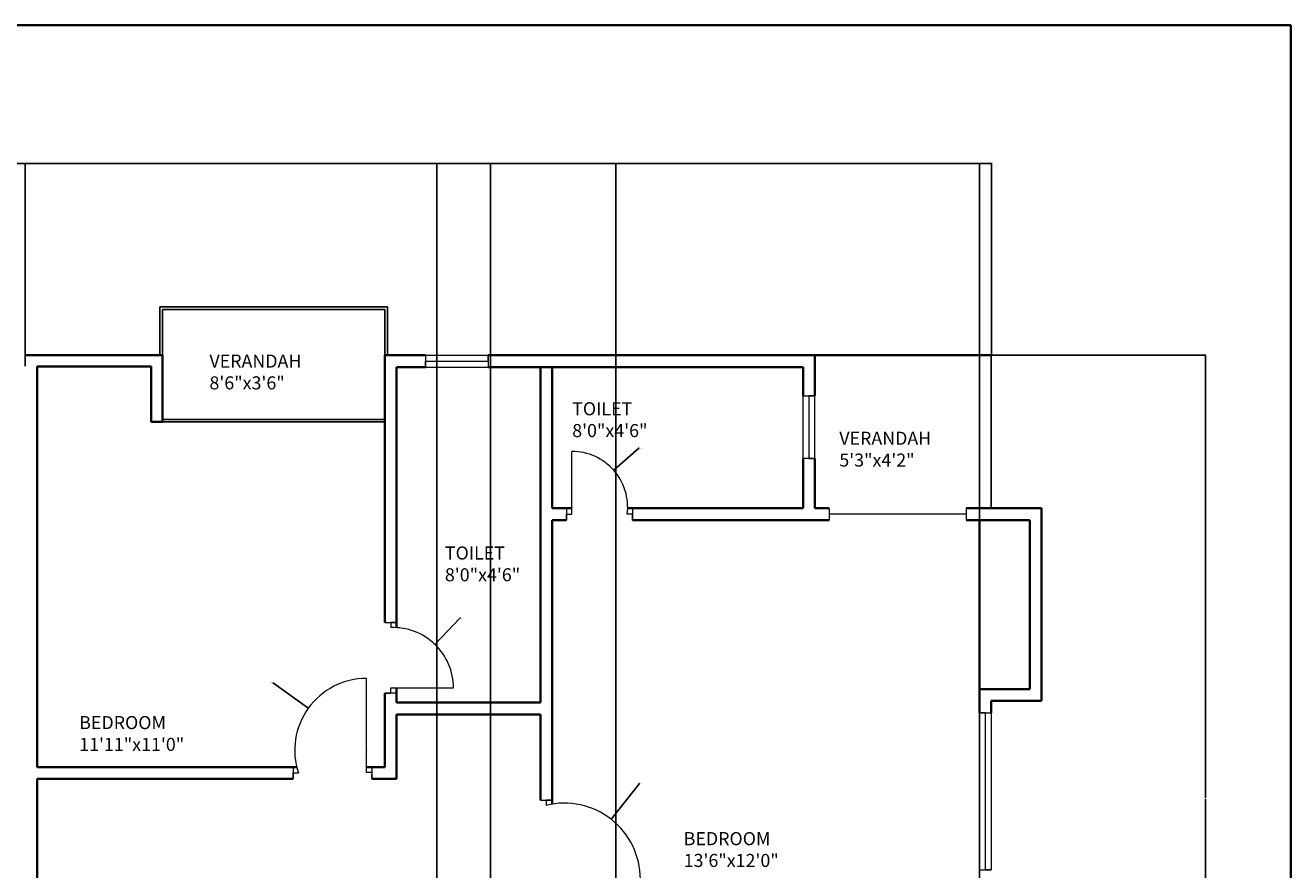
# Model space of a CAD drawing. Units: inches. Extents: x 2154 to 3131, y 1384 to 2688.
# Tile 5 of 5: x 2647 to 3131, y 2365 to 2688. Entities that reach past the tile are written whole.
import ezdxf

# ---------------------------------------------------------------- set-up
doc = ezdxf.new("R2010")
doc.units = ezdxf.units.IN
for name, color, linetype, lineweight in [('A-ANNO-DIMS', 2, 'Continuous', 18), ('A-ANNO-TTLB', 7, 'Continuous', 35), ('A-AREA-IDEN', 7, 'Continuous', 18), ('A-DOOR', 31, 'Continuous', 18), ('A-FLOR-BALC', 130, 'Continuous', 25), ('A-GLAZ', 130, 'Continuous', 18), ('A-WALL', 7, 'Continuous', 35)]:
    doc.layers.add(name, color=color, linetype=linetype, lineweight=lineweight)
doc.styles.get("Standard").update_dxf_attribs({"font": 'arial.ttf'})
doc.dimstyles.get("Standard").update_dxf_attribs({"dimtxt": 0.18, "dimasz": 0.18, "dimexe": 0.18, "dimexo": 0.0625, "dimgap": 0.09, "dimtad": 0, "dimtih": 1, "dimtoh": 1, "dimdec": 4, "dimzin": 0, "dimdsep": 46, "dimtxsty": 'Standard', "dimcen": 0.09, "dimadec": 0, "dimazin": 0, "dimtfac": 1, "dimtdec": 4, "dimtofl": 0, "dimtmove": 0, "dimatfit": 3, "dimfxl": 1, "dimtolj": 1, "dimtzin": 0, "dimarcsym": 0})

# ---------------------------------------------------------------- blocks, each defined once
blk = doc.blocks.new('DOOR-LEAF-24-JAMB-A')
for p, q in [((0, 2.25), (0, 26.25)), ((2, 2.25), (0, 2.25)), ((2, 4.5), (2, 0)), ((2, 0), (2, 2.25))]:
    blk.add_line(p, q)
blk = doc.blocks.new('WIN-24-FRAME-A')
for p, q in [((0, 4.5), (0, 0)), ((0, 4.5), (24, 4.5)), ((0, 0), (0, 2.25)), ((0, 2.25), (24, 2.25)), ((0, 0), (24, 0)), ((24, 2.25), (24, 4.5)), ((24, 4.5), (24, 0))]:
    blk.add_line(p, q)
blk = doc.blocks.new('WIN-60')
for p, q in [((2.25, 60), (0, 60)), ((0, 60), (4.5, 60)), ((0, 60), (0, 0)), ((2.25, 0), (2.25, 60)), ((4.5, 60), (4.5, 0)), ((0, 0), (4.5, 0)), ((4.5, 0), (2.25, 0))]:
    blk.add_line(p, q)
blk = doc.blocks.new('*D24')
at = {"layer": 'A-ANNO-DIMS', "color": 0, "lineweight": -2, "transparency": 16777216}
for p, q in [((2272.16, 2562.24), (2272.16, 2635.76)), ((2272.34, 2635.58), (2459.37, 2635.58)), ((2646.98, 2635.58), (2459.95, 2635.58)), ((2647.16, 2557.97), (2647.16, 2635.76))]:
    blk.add_line(p, q, dxfattribs=at)
at = {"layer": 'A-ANNO-DIMS', "color": 0, "transparency": 16777216}
for points in [[(2272.34, 2635.61), (2272.34, 2635.55), (2272.16, 2635.58)], [(2646.98, 2635.61), (2646.98, 2635.55), (2647.16, 2635.58)]]:
    blk.add_solid(points, dxfattribs=at)
at = {"layer": 'Defpoints', "color": 0, "transparency": 16777216}
for p in [(2647.16, 2635.58), (2272.16, 2562.18), (2647.16, 2557.91)]:
    blk.add_point(p, dxfattribs=at)
at = {"layer": 'A-ANNO-DIMS', "color": 0, "transparency": 16777216, "insert": (2459.66, 2635.58), "char_height": 0.18, "attachment_point": 5}
blk.add_mtext('\\A1;375', dxfattribs=at)
blk = doc.blocks.new('*D25')
at = {"layer": 'A-ANNO-DIMS', "color": 0, "lineweight": -2, "transparency": 16777216}
for p, q in [((2647.16, 2557.97), (2647.16, 2635.76)), ((2647.34, 2635.58), (2831.51, 2635.58)), ((3016.48, 2635.58), (2832.3, 2635.58)), ((3016.66, 2562.24), (3016.66, 2635.76))]:
    blk.add_line(p, q, dxfattribs=at)
at = {"layer": 'A-ANNO-DIMS', "color": 0, "transparency": 16777216}
for points in [[(2647.34, 2635.61), (2647.34, 2635.55), (2647.16, 2635.58)], [(3016.48, 2635.61), (3016.48, 2635.55), (3016.66, 2635.58)]]:
    blk.add_solid(points, dxfattribs=at)
at = {"layer": 'Defpoints', "color": 0, "transparency": 16777216}
for p in [(3016.66, 2635.58), (3016.66, 2562.18), (2647.16, 2557.91)]:
    blk.add_point(p, dxfattribs=at)
at = {"layer": 'A-ANNO-DIMS', "color": 0, "transparency": 16777216, "insert": (2831.91, 2635.58), "char_height": 0.18, "attachment_point": 5}
blk.add_mtext('\\A1;369.5', dxfattribs=at)
blk = doc.blocks.new('*D27')
at = {"layer": 'A-ANNO-DIMS', "color": 0, "lineweight": -2, "transparency": 16777216}
for p, q in [((2804.6, 2037.24), (2804.6, 2635.76)), ((2804.78, 2635.58), (2907.91, 2635.58)), ((3011.98, 2635.58), (2908.84, 2635.58)), ((3012.16, 2041.74), (3012.16, 2635.76))]:
    blk.add_line(p, q, dxfattribs=at)
at = {"layer": 'A-ANNO-DIMS', "color": 0, "transparency": 16777216}
for points in [[(2804.78, 2635.61), (2804.78, 2635.55), (2804.6, 2635.58)], [(3011.98, 2635.61), (3011.98, 2635.55), (3012.16, 2635.58)]]:
    blk.add_solid(points, dxfattribs=at)
at = {"layer": 'Defpoints', "color": 0, "transparency": 16777216}
for p in [(3012.16, 2635.58), (3012.16, 2041.68), (2804.6, 2037.18)]:
    blk.add_point(p, dxfattribs=at)
at = {"layer": 'A-ANNO-DIMS', "color": 0, "transparency": 16777216, "insert": (2908.38, 2635.58), "char_height": 0.18, "attachment_point": 5}
blk.add_mtext('\\A1;207.56', dxfattribs=at)
blk = doc.blocks.new('*D33')
at = {"layer": 'A-ANNO-DIMS', "color": 0, "lineweight": -2, "transparency": 16777216}
for p, q in [((3016.72, 2562.18), (3098.74, 2562.18)), ((3098.56, 2562), (3098.56, 2392.86)), ((3098.56, 2223.36), (3098.56, 2392.49)), ((2873.1, 2223.18), (3098.74, 2223.18))]:
    blk.add_line(p, q, dxfattribs=at)
at = {"layer": 'A-ANNO-DIMS', "color": 0, "transparency": 16777216}
for points in [[(3098.53, 2562), (3098.59, 2562), (3098.56, 2562.18)], [(3098.53, 2223.36), (3098.59, 2223.36), (3098.56, 2223.18)]]:
    blk.add_solid(points, dxfattribs=at)
at = {"layer": 'Defpoints', "color": 0, "transparency": 16777216}
for p in [(3016.66, 2562.18), (3098.56, 2562.18), (2873.04, 2223.18)]:
    blk.add_point(p, dxfattribs=at)
at = {"layer": 'A-ANNO-DIMS', "color": 0, "transparency": 16777216, "insert": (3098.56, 2392.68), "char_height": 0.18, "attachment_point": 5}
blk.add_mtext('\\A1;339', dxfattribs=at)
blk = doc.blocks.new('*D34')
at = {"layer": 'A-ANNO-DIMS', "color": 0, "lineweight": -2, "transparency": 16777216}
for p, q in [((2825.04, 2142.24), (2825.04, 2635.76)), ((2825.22, 2635.58), (2848.81, 2635.58)), ((2872.86, 2635.58), (2849.26, 2635.58)), ((2873.04, 2142.24), (2873.04, 2635.76))]:
    blk.add_line(p, q, dxfattribs=at)
at = {"layer": 'A-ANNO-DIMS', "color": 0, "transparency": 16777216}
for points in [[(2825.22, 2635.61), (2825.22, 2635.55), (2825.04, 2635.58)], [(2872.86, 2635.61), (2872.86, 2635.55), (2873.04, 2635.58)]]:
    blk.add_solid(points, dxfattribs=at)
at = {"layer": 'Defpoints', "color": 0, "transparency": 16777216}
for p in [(2873.04, 2635.58), (2825.04, 2142.18), (2873.04, 2142.18)]:
    blk.add_point(p, dxfattribs=at)
at = {"layer": 'A-ANNO-DIMS', "color": 0, "transparency": 16777216, "insert": (2849.04, 2635.58), "char_height": 0.18, "attachment_point": 5}
blk.add_mtext('\\A1;48', dxfattribs=at)
blk = doc.blocks.new('*D40')
at = {"layer": 'A-ANNO-DIMS', "color": 0, "lineweight": -2, "transparency": 16777216}
for p, q in [((2882.03, 2398.4), (2871.38, 2384.82)), ((2882.21, 2398.4), (2882.03, 2398.4)), ((2853.25, 2361.81), (2853.43, 2361.81)), ((2853.34, 2361.72), (2853.34, 2361.9))]:
    blk.add_line(p, q, dxfattribs=at)
at = {"layer": 'A-ANNO-DIMS', "color": 0, "transparency": 16777216}
blk.add_solid([(2871.36, 2384.84), (2871.41, 2384.8), (2871.27, 2384.68)], dxfattribs=at)
at = {"layer": 'Defpoints', "color": 0, "transparency": 16777216}
for p in [(2871.27, 2384.68), (2853.34, 2361.81)]:
    blk.add_point(p, dxfattribs=at)
at = {"layer": 'A-ANNO-DIMS', "color": 0, "transparency": 16777216, "insert": (2882.69, 2398.4), "char_height": 0.18, "attachment_point": 5}
blk.add_mtext('\\A1;R29.06', dxfattribs=at)
blk = doc.blocks.new('*D48')
at = {"layer": 'A-ANNO-DIMS', "color": 0, "lineweight": -2, "transparency": 16777216}
for p, q in [((2741.85, 2436.81), (2742.03, 2436.81)), ((2742.03, 2436.81), (2755.25, 2427.28)), ((2777.59, 2411.11), (2777.77, 2411.11)), ((2777.68, 2411.02), (2777.68, 2411.2))]:
    blk.add_line(p, q, dxfattribs=at)
at = {"layer": 'A-ANNO-DIMS', "color": 0, "transparency": 16777216}
blk.add_solid([(2755.27, 2427.3), (2755.23, 2427.25), (2755.4, 2427.17)], dxfattribs=at)
at = {"layer": 'Defpoints', "color": 0, "transparency": 16777216}
for p in [(2755.4, 2427.17), (2777.68, 2411.11)]:
    blk.add_point(p, dxfattribs=at)
at = {"layer": 'A-ANNO-DIMS', "color": 0, "transparency": 16777216, "insert": (2741.37, 2436.81), "char_height": 0.18, "attachment_point": 5}
blk.add_mtext('\\A1;R27.47', dxfattribs=at)
blk = doc.blocks.new('*D51')
at = {"layer": 'A-ANNO-DIMS', "color": 0, "lineweight": -2, "transparency": 16777216}
for p, q in [((2813.41, 2461.59), (2803.94, 2451.73)), ((2813.59, 2461.59), (2813.41, 2461.59)), ((2787.74, 2434.96), (2787.92, 2434.96)), ((2787.83, 2434.87), (2787.83, 2435.05))]:
    blk.add_line(p, q, dxfattribs=at)
at = {"layer": 'A-ANNO-DIMS', "color": 0, "transparency": 16777216}
blk.add_solid([(2803.92, 2451.75), (2803.96, 2451.71), (2803.82, 2451.6)], dxfattribs=at)
at = {"layer": 'Defpoints', "color": 0, "transparency": 16777216}
for p in [(2803.82, 2451.6), (2787.83, 2434.96)]:
    blk.add_point(p, dxfattribs=at)
at = {"layer": 'A-ANNO-DIMS', "color": 0, "transparency": 16777216, "insert": (2814.07, 2461.59), "char_height": 0.18, "attachment_point": 5}
blk.add_mtext('\\A1;R23.07', dxfattribs=at)
blk = doc.blocks.new('*D52')
at = {"layer": 'A-ANNO-DIMS', "color": 0, "lineweight": -2, "transparency": 16777216}
for p, q in [((2881.82, 2526.69), (2872.35, 2518.33)), ((2882, 2526.69), (2881.82, 2526.69)), ((2856.12, 2504.06), (2856.3, 2504.06)), ((2856.21, 2503.97), (2856.21, 2504.15))]:
    blk.add_line(p, q, dxfattribs=at)
at = {"layer": 'A-ANNO-DIMS', "color": 0, "transparency": 16777216}
blk.add_solid([(2872.33, 2518.35), (2872.37, 2518.3), (2872.22, 2518.21)], dxfattribs=at)
at = {"layer": 'Defpoints', "color": 0, "transparency": 16777216}
for p in [(2872.22, 2518.21), (2856.21, 2504.06)]:
    blk.add_point(p, dxfattribs=at)
at = {"layer": 'A-ANNO-DIMS', "color": 0, "transparency": 16777216, "insert": (2882.55, 2526.69), "char_height": 0.18, "attachment_point": 5}
blk.add_mtext('\\A1;R21.363', dxfattribs=at)

msp = doc.modelspace()

# ---------------------------------------------------------------- linework, layer by layer
at = {"layer": 'A-ANNO-TTLB'}
msp.add_lwpolyline([(2154.1953, 2688.4009), (3131.1627, 2688.4009), (3131.1627, 1383.7377), (2154.1953, 1383.7377)], close=True, dxfattribs=at)
at = {"layer": 'A-DOOR'}
for p, q in [((2879.4065, 2503.6767), (2879.4065, 2499.1767)), ((2879.4065, 2501.4267), (2877.4065, 2501.4267)), ((2879.4065, 2499.1767), (2879.4065, 2501.4267)), ((2784.656, 2460.0166), (2789.156, 2460.0166)), ((2789.156, 2460.0166), (2786.906, 2460.0166)), ((2786.906, 2460.0166), (2786.906, 2458.0166)), ((2777.6787, 2402.5782), (2777.6787, 2438.5782)), ((2749.6151, 2404.6767), (2749.6151, 2400.1767)), ((2749.6151, 2400.1767), (2749.6151, 2402.4267)), ((2749.6151, 2402.4267), (2751.6151, 2402.4267)), ((2779.6787, 2402.5782), (2777.6787, 2402.5782)), ((2779.6787, 2404.6767), (2779.6787, 2401.8703)), ((2779.6787, 2401.8703), (2779.6787, 2400.1767)), ((2779.6787, 2400.1767), (2779.6787, 2401.8703)), ((2844.156, 2392.0311), (2848.656, 2392.0311)), ((2848.656, 2392.0311), (2846.406, 2392.0311)), ((2846.406, 2392.0311), (2846.406, 2390.0311))]:
    msp.add_line(p, q, dxfattribs=at)
for centre, radius, start, end in [((2856.2066, 2504.0634), 21.3633, 352.910373, 90), ((2787.8343, 2434.9635), 23.0717, 0, 92.305849), ((2777.6787, 2411.1071), 27.4711, 90, 198.42019), ((2853.3445, 2361.81), 29.0615, 360, 103.812872)]:
    msp.add_arc(centre, radius, start, end, dxfattribs=at)
at = {"layer": 'A-FLOR-BALC'}
for p, q in [((2698.656, 2580.6767), (2785.656, 2580.6767)), ((2699.656, 2580.6767), (2698.656, 2580.6767)), ((2698.656, 2580.6767), (2698.656, 2562.1767)), ((2785.656, 2580.6767), (2785.656, 2562.1767)), ((2784.656, 2579.6767), (2699.656, 2579.6767)), ((2699.656, 2562.1767), (2699.656, 2579.6767)), ((2784.656, 2562.1767), (2784.656, 2579.6767)), ((3016.656, 2562.1767), (3016.656, 2557.6767)), ((3016.656, 2557.6767), (3016.656, 2503.6767)), ((2699.6214, 2537.6767), (2784.656, 2537.6767)), ((2784.656, 2536.6767), (2699.6214, 2536.6767))]:
    msp.add_line(p, q, dxfattribs=at)
at = {"layer": 'A-GLAZ'}
for p, q in [((2944.656, 2546.6596), (2949.156, 2546.6596)), ((2944.656, 2522.6596), (2944.656, 2546.6596)), ((2949.156, 2546.6596), (2946.906, 2546.6596)), ((2946.906, 2546.6596), (2946.906, 2522.6596)), ((2949.156, 2524.1377), (2949.156, 2546.6596)), ((2949.156, 2522.6596), (2944.656, 2522.6596)), ((2946.906, 2522.6596), (2949.156, 2522.6596)), ((2949.156, 2522.6596), (2949.156, 2524.1377)), ((2954.5972, 2503.6767), (2954.5972, 2499.1767)), ((3007.0846, 2503.6767), (3007.0846, 2499.1767)), ((3007.0846, 2501.4267), (2954.5972, 2501.4267))]:
    msp.add_line(p, q, dxfattribs=at)
at = {"layer": 'A-WALL'}
for p, q in [((2647.156, 2562.1767), (2699.656, 2562.1767)), ((2699.656, 2536.6767), (2699.656, 2562.1767)), ((2784.656, 2562.1767), (2784.656, 2460.0166)), ((2784.656, 2562.1767), (2800.2388, 2562.1767)), ((2824.2388, 2562.1767), (3016.656, 2562.1767)), ((2949.156, 2562.1767), (2949.156, 2546.6596)), ((2651.656, 2557.9062), (2651.656, 2404.6767)), ((2651.656, 2557.9062), (2695.2402, 2557.9062)), ((2695.2402, 2557.9062), (2695.2402, 2536.6767)), ((2789.156, 2557.6767), (2789.156, 2457.9974)), ((2789.156, 2557.6767), (2800.2388, 2557.6767)), ((2824.2388, 2557.6767), (2944.656, 2557.6767)), ((2844.156, 2557.6767), (2844.156, 2429.312)), ((2848.656, 2557.6767), (2848.656, 2503.6767)), ((2944.656, 2557.6767), (2944.656, 2546.6596)), ((2695.2402, 2536.6767), (2696.952, 2536.6767)), ((2696.7402, 2536.6767), (2699.656, 2536.6767)), ((2944.656, 2522.6596), (2944.656, 2503.6767)), ((2949.156, 2522.6596), (2949.156, 2503.6767)), ((2848.656, 2503.6767), (2856.2066, 2503.6767)), ((2877.5664, 2503.6767), (2944.656, 2503.6767)), ((2949.156, 2503.6767), (2954.5972, 2503.6767)), ((3007.0846, 2503.6767), (3016.656, 2503.6767)), ((3011.8703, 2503.6767), (3035.8703, 2503.6767)), ((3035.8703, 2503.6767), (3035.8703, 2430.0303)), ((2848.656, 2499.1767), (2854.2066, 2499.1767)), ((2848.656, 2499.1767), (2848.656, 2390.4908)), ((2879.4065, 2499.1767), (2954.5972, 2499.1767)), ((3007.0846, 2499.1767), (3012.156, 2499.1767)), ((3012.156, 2499.1767), (3031.3703, 2499.1767)), ((3012.156, 2434.5303), (3012.156, 2499.1767)), ((3031.3703, 2499.1767), (3031.3703, 2434.5303)), ((2789.156, 2434.9635), (2789.156, 2429.312)), ((2784.656, 2432.9635), (2784.656, 2404.6767)), ((3031.3703, 2434.5303), (3012.156, 2434.5303)), ((3012.156, 2434.5303), (3012.156, 2430.0303)), ((3012.156, 2430.0303), (3012.156, 2425.4173)), ((3035.8703, 2430.0303), (3016.656, 2430.0303)), ((3016.656, 2430.0303), (3016.656, 2425.4173)), ((2789.156, 2429.312), (2844.156, 2429.312)), ((2789.156, 2424.812), (2844.156, 2424.812)), ((2789.156, 2424.812), (2789.156, 2400.1767)), ((2844.156, 2424.812), (2844.156, 2392.0311)), ((2651.656, 2404.6767), (2750.9708, 2404.6767)), ((2777.6787, 2404.6767), (2784.656, 2404.6767)), ((2749.6151, 2400.1767), (2651.656, 2400.1767)), ((2651.656, 2400.1767), (2651.656, 2142.1767)), ((2789.156, 2400.1767), (2779.6787, 2400.1767))]:
    msp.add_line(p, q, dxfattribs=at)

# ---------------------------------------------------------------- block references
at = {"layer": 'A-DOOR', "extrusion": (0, 0, -1), "zscale": -1}
msp.add_blockref('DOOR-LEAF-24-JAMB-A', (-2856.2066, 2499.1767), dxfattribs=at)
at = {"layer": 'A-DOOR', "rotation": 270.0000000000001}
msp.add_blockref('DOOR-LEAF-24-JAMB-A', (2784.656, 2434.9635), dxfattribs=at)
at = {"layer": 'A-GLAZ'}
for name, p in [('WIN-24-FRAME-A', (2800.2388, 2557.6767)), ('WIN-60', (3012.156, 2365.4173))]:
    msp.add_blockref(name, p, dxfattribs=at)

# ---------------------------------------------------------------- texts
at = {"layer": 'A-AREA-IDEN', "char_height": 5, "attachment_point": 1}
for s, width, insert in [('VERANDAH\\P8\'6"x3\'6"', 127.045563, (2717.5948, 2562.4636)), ('TOILET\\P8\'0"x4\'6"', 134.909081, (2856.3471, 2544.2149)), ('VERANDAH\\P5\'3"x4\'2"', 89.073942, (2958.5116, 2532.9432)), ('TOILET\\P8\'0"x4\'6"', 188.441463, (2807.6484, 2489.0603)), ('BEDROOM\\P11\'11"x11\'0"', 221.791605, (2667.78, 2424.1801)), ('BEDROOM\\P13\'6"x12\'0"', 226.623566, (2898.9803, 2379.79))]:
    msp.add_mtext_dynamic_manual_height_columns(s, width=width, gutter_width=12.5, heights=[0], dxfattribs=dict(at, insert=insert))

# ---------------------------------------------------------------- dimensions: what is measured, and where the dimension line sits
at = {"layer": 'A-ANNO-DIMS'}
for base, p1, p2, override, picture, middle in [((2647.156, 2635.5767), (2272.156, 2562.1767), (2647.156, 2557.9062), {"dimdec": 0, "dimlfac": 1, "dimrnd": 0, "dimzin": 0, "dimdsep": 46, "dimlunit": 2}, '*D24', (2459.656, 2635.5767)), ((3016.656, 2635.5767), (2647.156, 2557.9062), (3016.656, 2562.1767), {"dimdec": 1, "dimlfac": 1, "dimrnd": 0, "dimzin": 0, "dimdsep": 46, "dimlunit": 2}, '*D25', (2831.906, 2635.5767)), ((3012.156, 2635.5767), (2804.5995, 2037.1767), (3012.156, 2041.6767), {"dimdec": 2, "dimlfac": 1, "dimrnd": 0, "dimzin": 0, "dimdsep": 46, "dimlunit": 2}, '*D27', (2908.3778, 2635.5767)), ((2873.0368, 2635.5767), (2825.0368, 2142.1767), (2873.0368, 2142.1767), {"dimdec": 0, "dimlfac": 1, "dimrnd": 0, "dimzin": 0, "dimdsep": 46, "dimlunit": 2}, '*D34', (2849.0368, 2635.5767))]:
    dim = msp.add_linear_dim(base=base, p1=p1, p2=p2, dimstyle='Standard', override=override, dxfattribs=at)
    dim.commit()
    dim.dimension.update_dxf_attribs({"geometry": picture, "text_midpoint": middle})
dim = msp.add_linear_dim(base=(3098.556, 2562.1767), p1=(2873.0368, 2223.1767), p2=(3016.656, 2562.1767), angle=90, dimstyle='Standard', override={"dimdec": 0, "dimlfac": 1, "dimrnd": 0, "dimzin": 0, "dimdsep": 46, "dimlunit": 2}, dxfattribs=at)
dim.commit()
dim.dimension.update_dxf_attribs({"geometry": '*D33', "text_midpoint": (3098.556, 2392.6767)})
for center, mpoint, override, picture, middle in [((2856.2066, 2504.0634), (2872.2177, 2518.2067), {"dimdec": 3, "dimlfac": 1, "dimrnd": 0, "dimzin": 0, "dimdsep": 46, "dimlunit": 2}, '*D52', (2882.5541, 2526.6927)), ((2787.8343, 2434.9635), (2803.8168, 2451.6028), {"dimdec": 2, "dimlfac": 1, "dimrnd": 0, "dimzin": 0, "dimdsep": 46, "dimlunit": 2}, '*D51', (2814.0661, 2461.5863)), ((2777.6787, 2411.1071), (2755.3952, 2427.1729), {"dimdec": 2, "dimlfac": 1, "dimrnd": 0, "dimzin": 0, "dimdsep": 46, "dimlunit": 2}, '*D48', (2741.3653, 2436.8123)), ((2853.3445, 2361.81), (2871.2737, 2384.6817), {"dimdec": 2, "dimlfac": 1, "dimrnd": 0, "dimzin": 0, "dimdsep": 46, "dimlunit": 2}, '*D40', (2882.6911, 2398.4047))]:
    dim = msp.add_radius_dim(center=center, mpoint=mpoint, dimstyle='Standard', override=override, dxfattribs=at)
    dim.commit()
    dim.dimension.update_dxf_attribs({"geometry": picture, "text_midpoint": middle, "dimtype": 164})

doc.saveas('drawing.dxf')
